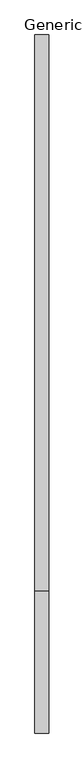
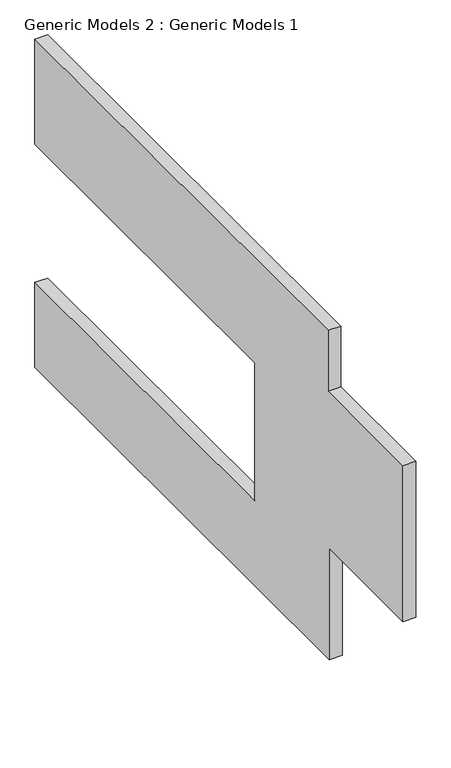
"""IFC4 building model written with IfcOpenShell, lengths in millimetres: proxy geometry, Generic Models 2 : Generic Models 1."""

from ifc_helpers import new_model, si_unit, frame, origin, place, context, project, spatial, polyline, outline, extrude, source, transform, mapped, element, save


def generic_models_2_generic_models_1_28cf7cb4(model_context):
    return source(origin(), model_context, "Body", "SweptSolid", [
        extrude(outline(polyline([(-3946.8023495, -577.85), (-3946.8023495, 2214.7139463), (-6979.1363705, 2214.7139463), (-6979.1363705, 6127.75), (-3899.3863708, 6127.75), (-3899.3863708, 7651.75), (8140.2136292, 7651.75), (8140.2136292, 5015.8429185), (-883.1363705, 5015.8429185), (-883.1363705, 1555.75), (8140.2136292, 1555.75), (8140.2136292, -577.85), (-3946.8023495, -577.85)])), frame((13902.5156363, 0.0, 0.0), z_axis=(1.0, 0.0, 0.0), x_axis=(0.0, 1.0, 0.0)), (0.0, 0.0, 1.0), 304.8),
    ])


if __name__ == "__main__":
    model = new_model("IFC4")
    model_context = context("Model", 3, world=origin())
    ifc_project = project(units=[si_unit("LENGTHUNIT", "METRE", prefix="MILLI")], contexts=[model_context])
    site = spatial("IfcSite", under=ifc_project)
    building = spatial("IfcBuilding", under=site)
    placement = place(None, origin())
    generic_models_2_generic_models_1_shape = generic_models_2_generic_models_1_28cf7cb4(model_context)
    element("IfcBuildingElementProxy", 1, Name="Generic Models 2 : Generic Models 1", ObjectType="Generic Models 2 : Generic Models 1", at=placement, inside=building, context=model_context, shape_type="MappedRepresentation", body=[
        mapped(generic_models_2_generic_models_1_shape, transform((0.0, 0.0, 0.0), x_axis=(1.0, 0.0, 0.0), y_axis=(0.0, 1.0, 0.0), z_axis=(0.0, 0.0, 1.0))),
    ])
    save(model, "model.ifc")
